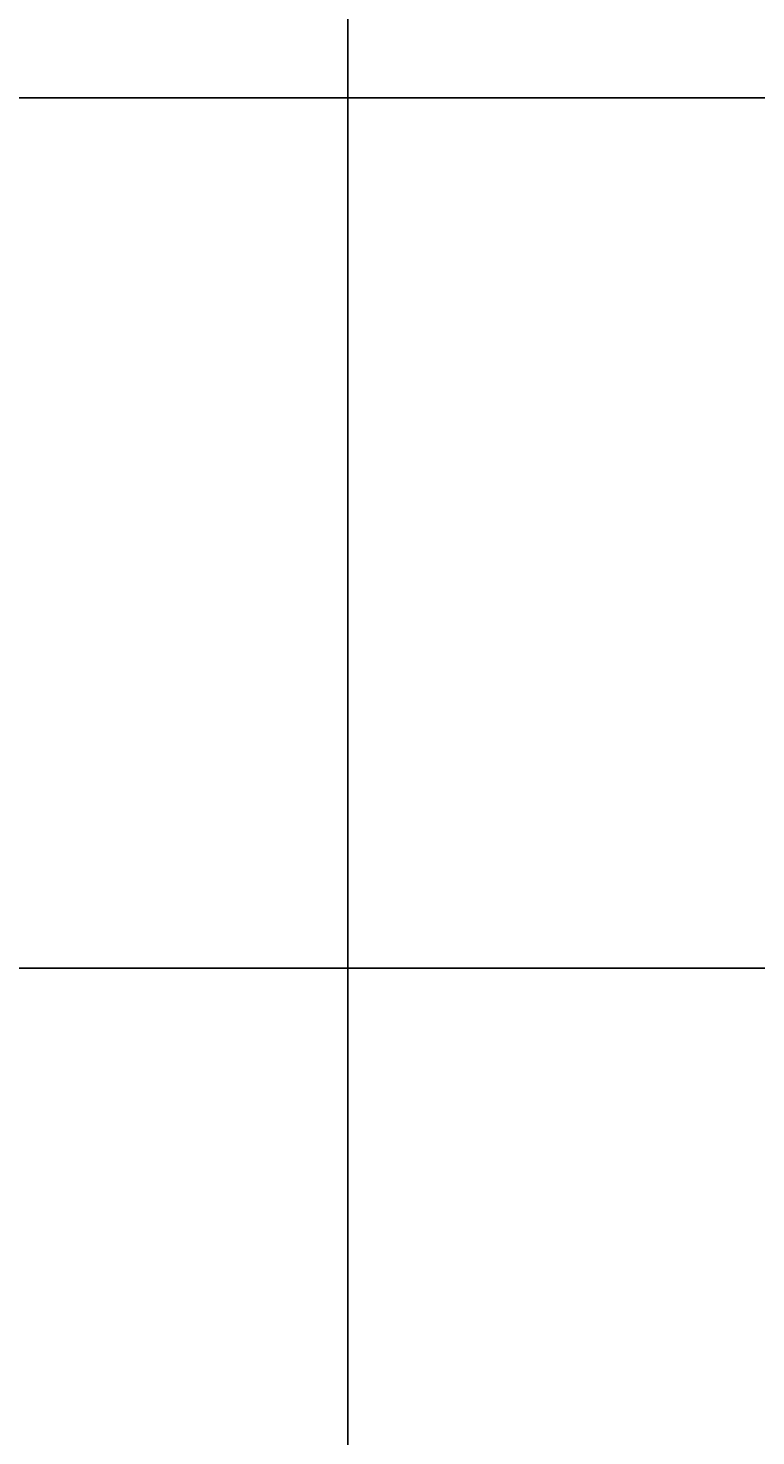
# Model space of a CAD drawing. Units: inches. Extents: x 502 to 1235, y -850 to 110.
# Tile 5 of 9: x 867 to 931, y -335 to -212. Entities that reach past the tile are written whole.
import ezdxf

# ---------------------------------------------------------------- set-up
doc = ezdxf.new("R2010")
doc.units = ezdxf.units.IN
doc.header["$MEASUREMENT"] = 0
doc.layers.add('A-ANNO-DIMS', color=2, linetype='Continuous', lineweight=18)
doc.styles.get("Standard").update_dxf_attribs({"font": 'arial.ttf'})
doc.dimstyles.get("Standard").update_dxf_attribs({"dimtxt": 0.18, "dimasz": 0.18, "dimexe": 0.18, "dimexo": 0.0625, "dimgap": 0.09, "dimtad": 0, "dimtih": 1, "dimtoh": 1, "dimdec": 1, "dimzin": 0, "dimdsep": 46, "dimlunit": 4, "dimtxsty": 'Standard', "dimcen": 0.09, "dimadec": 0, "dimazin": 0, "dimtfac": 1, "dimtdec": 1, "dimtofl": 0, "dimtmove": 0, "dimatfit": 3, "dimfxl": 1, "dimtolj": 1, "dimtzin": 0, "dimarcsym": 0})

# ---------------------------------------------------------------- blocks, each defined once
blk = doc.blocks.new('*D25')
at = {"layer": 'A-ANNO-DIMS', "color": 0, "lineweight": -2, "transparency": 16777216}
for p, q in [((798.89, -699.78), (798.89, 63.98)), ((799.07, 63.8), (846.56, 63.8)), ((894.71, 63.8), (847.22, 63.8)), ((894.89, -699.78), (894.89, 63.98))]:
    blk.add_line(p, q, dxfattribs=at)
at = {"layer": 'A-ANNO-DIMS', "color": 0, "transparency": 16777216}
for points in [[(799.07, 63.83), (799.07, 63.77), (798.89, 63.8)], [(894.71, 63.83), (894.71, 63.77), (894.89, 63.8)]]:
    blk.add_solid(points, dxfattribs=at)
at = {"layer": 'Defpoints', "color": 0, "transparency": 16777216}
for p in [(894.89, 63.8), (798.89, -699.85), (894.89, -699.85)]:
    blk.add_point(p, dxfattribs=at)
at = {"layer": 'A-ANNO-DIMS', "color": 0, "transparency": 16777216, "insert": (846.89, 63.8), "char_height": 0.18, "attachment_point": 5}
blk.add_mtext('\\A1;8\'-0"', dxfattribs=at)
blk = doc.blocks.new('*D28')
at = {"layer": 'A-ANNO-DIMS', "color": 0, "lineweight": -2, "transparency": 16777216}
for p, q in [((770.85, -217.85), (1235.01, -217.85)), ((1234.83, -218.03), (1234.83, -255.91)), ((1234.83, -294.17), (1234.83, -256.28)), ((770.85, -294.35), (1235.01, -294.35))]:
    blk.add_line(p, q, dxfattribs=at)
at = {"layer": 'A-ANNO-DIMS', "color": 0, "transparency": 16777216}
for points in [[(1234.8, -218.03), (1234.86, -218.03), (1234.83, -217.85)], [(1234.8, -294.17), (1234.86, -294.17), (1234.83, -294.35)]]:
    blk.add_solid(points, dxfattribs=at)
at = {"layer": 'Defpoints', "color": 0, "transparency": 16777216}
for p in [(770.79, -217.85), (770.79, -294.35), (1234.83, -294.35)]:
    blk.add_point(p, dxfattribs=at)
at = {"layer": 'A-ANNO-DIMS', "color": 0, "transparency": 16777216, "insert": (1234.83, -256.1), "char_height": 0.18, "attachment_point": 5}
blk.add_mtext('\\A1;6\'-4 1/2"', dxfattribs=at)
blk = doc.blocks.new('*D29')
at = {"layer": 'A-ANNO-DIMS', "color": 0, "lineweight": -2, "transparency": 16777216}
for p, q in [((644.45, -193.85), (1235.01, -193.85)), ((1234.83, -194.03), (1234.83, -205.66)), ((1234.83, -217.67), (1234.83, -206.03)), ((644.45, -217.85), (1235.01, -217.85))]:
    blk.add_line(p, q, dxfattribs=at)
at = {"layer": 'A-ANNO-DIMS', "color": 0, "transparency": 16777216}
for points in [[(1234.8, -194.03), (1234.86, -194.03), (1234.83, -193.85)], [(1234.8, -217.67), (1234.86, -217.67), (1234.83, -217.85)]]:
    blk.add_solid(points, dxfattribs=at)
at = {"layer": 'Defpoints', "color": 0, "transparency": 16777216}
for p in [(644.39, -193.85), (644.39, -217.85), (1234.83, -217.85)]:
    blk.add_point(p, dxfattribs=at)
at = {"layer": 'A-ANNO-DIMS', "color": 0, "transparency": 16777216, "insert": (1234.83, -205.85), "char_height": 0.18, "attachment_point": 5}
blk.add_mtext('\\A1;2\'-0"', dxfattribs=at)

msp = doc.modelspace()

# ---------------------------------------------------------------- dimensions: what is measured, and where the dimension line sits
at = {"layer": 'A-ANNO-DIMS'}
dim = msp.add_linear_dim(base=(894.89, 63.8), p1=(798.89, -699.85), p2=(894.89, -699.85), dimstyle='Standard', override={"dimdec": 1, "dimlfac": 1, "dimrnd": 0, "dimzin": 1, "dimdsep": 46, "dimlunit": 4, "dimfrac": 2}, dxfattribs=at)
dim.commit()
dim.dimension.update_dxf_attribs({"geometry": '*D25', "text_midpoint": (846.89, 63.8)})
for base, p1, p2, picture, middle in [((1234.83, -217.85), (644.39, -193.85), (644.39, -217.85), '*D29', (1234.83, -205.85)), ((1234.83, -294.35), (770.79, -217.85), (770.79, -294.35), '*D28', (1234.83, -256.1))]:
    dim = msp.add_linear_dim(base=base, p1=p1, p2=p2, angle=90, dimstyle='Standard', override={"dimdec": 1, "dimlfac": 1, "dimrnd": 0, "dimzin": 1, "dimdsep": 46, "dimlunit": 4, "dimfrac": 2}, dxfattribs=at)
    dim.commit()
    dim.dimension.update_dxf_attribs({"geometry": picture, "text_midpoint": middle})

doc.saveas('drawing.dxf')
